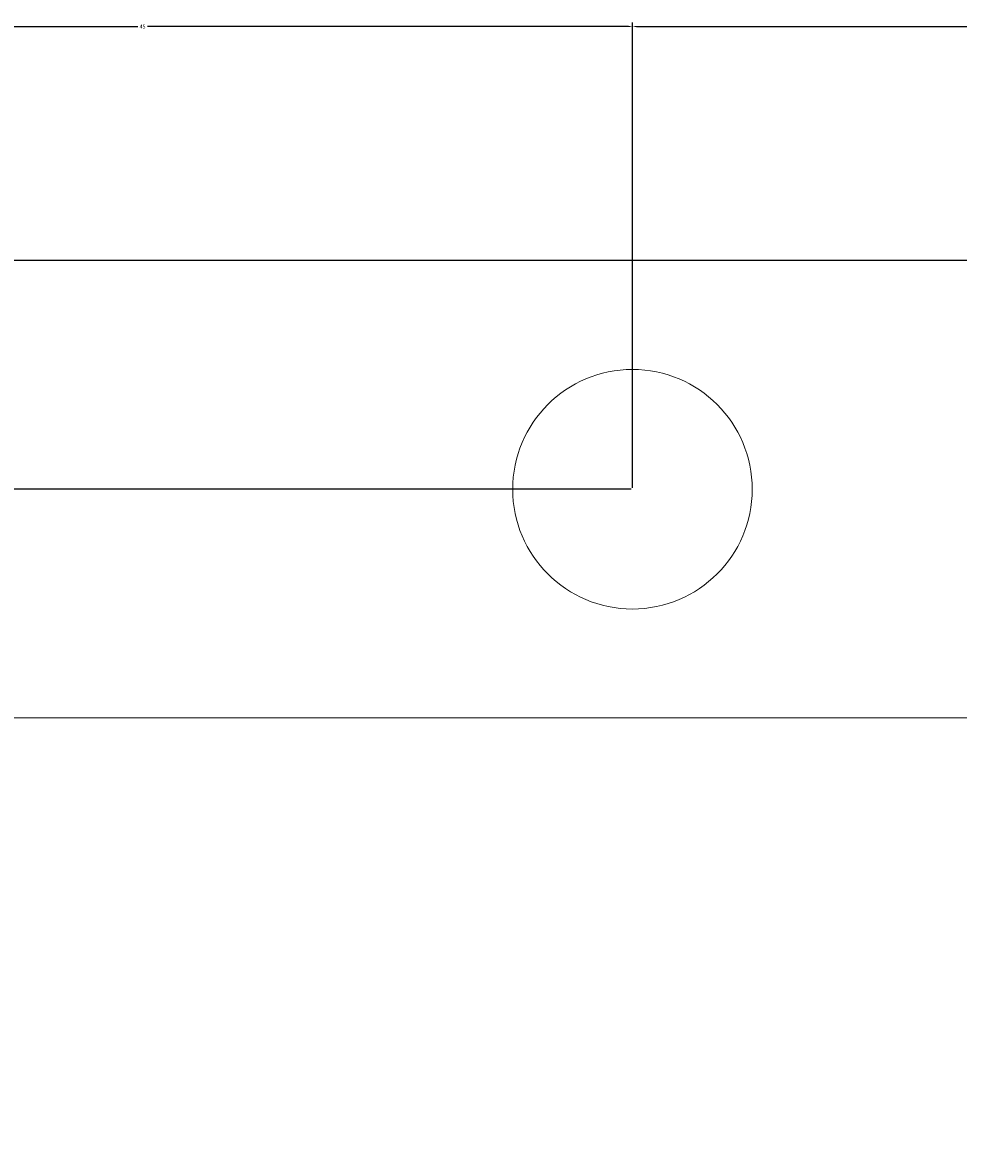
# Model space of a CAD drawing. Units: millimetres. Extents: x 315 to 487, y -72 to 32.
# Tile 3 of 4: x 358 to 401, y -20 to 32. Entities that reach past the tile are written whole.
import ezdxf

# ---------------------------------------------------------------- set-up
doc = ezdxf.new("R2010")
doc.units = ezdxf.units.MM
doc.layers.add('M-CONS', color=8, linetype='Continuous', lineweight=13)
doc.layers.add('M-DIMS', color=2, linetype='Continuous', lineweight=18)
doc.styles.get("Standard").update_dxf_attribs({"font": 'arial.ttf'})
doc.dimstyles.get("Standard").update_dxf_attribs({"dimtxt": 0.18, "dimasz": 0.18, "dimexe": 0.18, "dimexo": 0.0625, "dimgap": 0.09, "dimtad": 0, "dimtih": 1, "dimtoh": 1, "dimdec": 4, "dimzin": 0, "dimdsep": 46, "dimtxsty": 'Standard', "dimcen": 0.09, "dimadec": 0, "dimazin": 0, "dimtfac": 1, "dimtdec": 4, "dimtofl": 0, "dimtmove": 0, "dimatfit": 3, "dimfxl": 1, "dimtolj": 1, "dimtzin": 0, "dimarcsym": 0})

# ---------------------------------------------------------------- blocks, each defined once
blk = doc.blocks.new('*D3')
at = {"layer": 'Defpoints', "color": 0, "transparency": 16777216}
for p in [(326.007, 0), (476.007, 0), (476.007, -71.75)]:
    blk.add_point(p, dxfattribs=at)
at = {"layer": 'M-DIMS', "color": 0, "lineweight": -2, "transparency": 16777216}
for p, q in [((326.007, -0.062), (326.007, -71.93)), ((476.007, -0.062), (476.007, -71.93)), ((326.187, -71.75), (400.727, -71.75)), ((475.827, -71.75), (401.287, -71.75))]:
    blk.add_line(p, q, dxfattribs=at)
at = {"layer": 'M-DIMS', "color": 0, "transparency": 16777216}
for points in [[(326.187, -71.72), (326.187, -71.78), (326.007, -71.75)], [(475.827, -71.72), (475.827, -71.78), (476.007, -71.75)]]:
    blk.add_solid(points, dxfattribs=at)
at = {"layer": 'M-DIMS', "color": 0, "transparency": 16777216, "insert": (401.007, -71.75), "char_height": 0.18, "attachment_point": 5}
blk.add_mtext('\\A1;150', dxfattribs=at)
blk = doc.blocks.new('*D6')
at = {"layer": 'Defpoints', "color": 0, "transparency": 16777216}
for p in [(386.007, 31.75), (386.007, 10.5), (341.007, 0)]:
    blk.add_point(p, dxfattribs=at)
at = {"layer": 'M-DIMS', "color": 0, "lineweight": -2, "transparency": 16777216}
for p, q in [((341.007, 0.062), (341.007, 31.93)), ((341.187, 31.75), (363.284, 31.75)), ((385.827, 31.75), (363.731, 31.75)), ((386.007, 10.562), (386.007, 31.93))]:
    blk.add_line(p, q, dxfattribs=at)
at = {"layer": 'M-DIMS', "color": 0, "transparency": 16777216}
for points in [[(341.187, 31.78), (341.187, 31.72), (341.007, 31.75)], [(385.827, 31.78), (385.827, 31.72), (386.007, 31.75)]]:
    blk.add_solid(points, dxfattribs=at)
at = {"layer": 'M-DIMS', "color": 0, "transparency": 16777216, "insert": (363.507, 31.75), "char_height": 0.18, "attachment_point": 5}
blk.add_mtext('\\A1;45', dxfattribs=at)
blk = doc.blocks.new('*D7')
at = {"layer": 'Defpoints', "color": 0, "transparency": 16777216}
for p in [(446.007, 31.75), (386.007, 10.5), (446.007, 10.5)]:
    blk.add_point(p, dxfattribs=at)
at = {"layer": 'M-DIMS', "color": 0, "lineweight": -2, "transparency": 16777216}
for p, q in [((386.007, 10.562), (386.007, 31.93)), ((386.187, 31.75), (415.788, 31.75)), ((445.827, 31.75), (416.227, 31.75)), ((446.007, 10.562), (446.007, 31.93))]:
    blk.add_line(p, q, dxfattribs=at)
at = {"layer": 'M-DIMS', "color": 0, "transparency": 16777216}
for points in [[(386.187, 31.78), (386.187, 31.72), (386.007, 31.75)], [(445.827, 31.78), (445.827, 31.72), (446.007, 31.75)]]:
    blk.add_solid(points, dxfattribs=at)
at = {"layer": 'M-DIMS', "color": 0, "transparency": 16777216, "insert": (416.007, 31.75), "char_height": 0.18, "attachment_point": 5}
blk.add_mtext('\\A1;60', dxfattribs=at)
blk = doc.blocks.new('*D11')
at = {"layer": 'Defpoints', "color": 0, "transparency": 16777216}
for p in [(315.257, 10.5), (386.007, 10.5), (326.007, 0)]:
    blk.add_point(p, dxfattribs=at)
at = {"layer": 'M-DIMS', "color": 0, "lineweight": -2, "transparency": 16777216}
for p, q in [((385.945, 10.5), (315.077, 10.5)), ((315.257, 10.32), (315.257, 5.432)), ((315.257, 0.18), (315.257, 5.068)), ((325.945, 0), (315.077, 0))]:
    blk.add_line(p, q, dxfattribs=at)
at = {"layer": 'M-DIMS', "color": 0, "transparency": 16777216}
for points in [[(315.227, 10.32), (315.287, 10.32), (315.257, 10.5)], [(315.227, 0.18), (315.287, 0.18), (315.257, 0)]]:
    blk.add_solid(points, dxfattribs=at)
at = {"layer": 'M-DIMS', "color": 0, "transparency": 16777216, "insert": (315.257, 5.25), "char_height": 0.18, "attachment_point": 5}
blk.add_mtext('\\A1;10.5', dxfattribs=at)
blk = doc.blocks.new('*D12')
at = {"layer": 'Defpoints', "color": 0, "transparency": 16777216}
for p in [(315.257, 21), (446.007, 21), (386.007, 10.5)]:
    blk.add_point(p, dxfattribs=at)
at = {"layer": 'M-DIMS', "color": 0, "lineweight": -2, "transparency": 16777216}
for p, q in [((445.945, 21), (315.077, 21)), ((315.257, 20.82), (315.257, 15.932)), ((315.257, 10.68), (315.257, 15.568)), ((385.945, 10.5), (315.077, 10.5))]:
    blk.add_line(p, q, dxfattribs=at)
at = {"layer": 'M-DIMS', "color": 0, "transparency": 16777216}
for points in [[(315.227, 20.82), (315.287, 20.82), (315.257, 21)], [(315.227, 10.68), (315.287, 10.68), (315.257, 10.5)]]:
    blk.add_solid(points, dxfattribs=at)
at = {"layer": 'M-DIMS', "color": 0, "transparency": 16777216, "insert": (315.257, 15.75), "char_height": 0.18, "attachment_point": 5}
blk.add_mtext('\\A1;10.5', dxfattribs=at)

msp = doc.modelspace()

# ---------------------------------------------------------------- linework, layer by layer
at = {"layer": 'M-CONS', "extrusion": (0, -1, 0)}
for p, q in [((326.007, 0, 190.054), (476.007, 0, 190.054)), ((466.007, 0, 200.054), (326.007, 0, 200.054)), ((434.007, 0, 240.054), (338.273, 0, 222.303))]:
    msp.add_line(p, q, dxfattribs=at)
at = {"layer": 'M-CONS'}
msp.add_circle((386.007, 10.5, 200.054), 5.5, dxfattribs=at)

# ---------------------------------------------------------------- dimensions: what is measured, and where the dimension line sits
at = {"layer": 'M-DIMS'}
for base, p1, p2, picture, middle in [((386.007, 31.75), (341.007, 0), (386.007, 10.5), '*D6', (363.507, 31.75)), ((446.007, 31.75), (386.007, 10.5), (446.007, 10.5), '*D7', (416.007, 31.75)), ((476.007, -71.75), (326.007, 0), (476.007, 0), '*D3', (401.007, -71.75))]:
    dim = msp.add_linear_dim(base=base, p1=p1, p2=p2, dimstyle='Standard', override={"dimdec": 0, "dimlfac": 1, "dimrnd": 0, "dimzin": 0, "dimdsep": 46, "dimlunit": 2}, dxfattribs=at)
    dim.commit()
    dim.dimension.update_dxf_attribs({"geometry": picture, "text_midpoint": middle})
for base, p1, p2, picture, middle in [((315.257, 21), (386.007, 10.5), (446.007, 21), '*D12', (315.257, 15.75)), ((315.257, 10.5), (326.007, 0), (386.007, 10.5), '*D11', (315.257, 5.25))]:
    dim = msp.add_linear_dim(base=base, p1=p1, p2=p2, angle=90, dimstyle='Standard', override={"dimdec": 1, "dimlfac": 1, "dimrnd": 0, "dimzin": 0, "dimdsep": 46, "dimlunit": 2}, dxfattribs=at)
    dim.commit()
    dim.dimension.update_dxf_attribs({"geometry": picture, "text_midpoint": middle})

doc.saveas('drawing.dxf')
